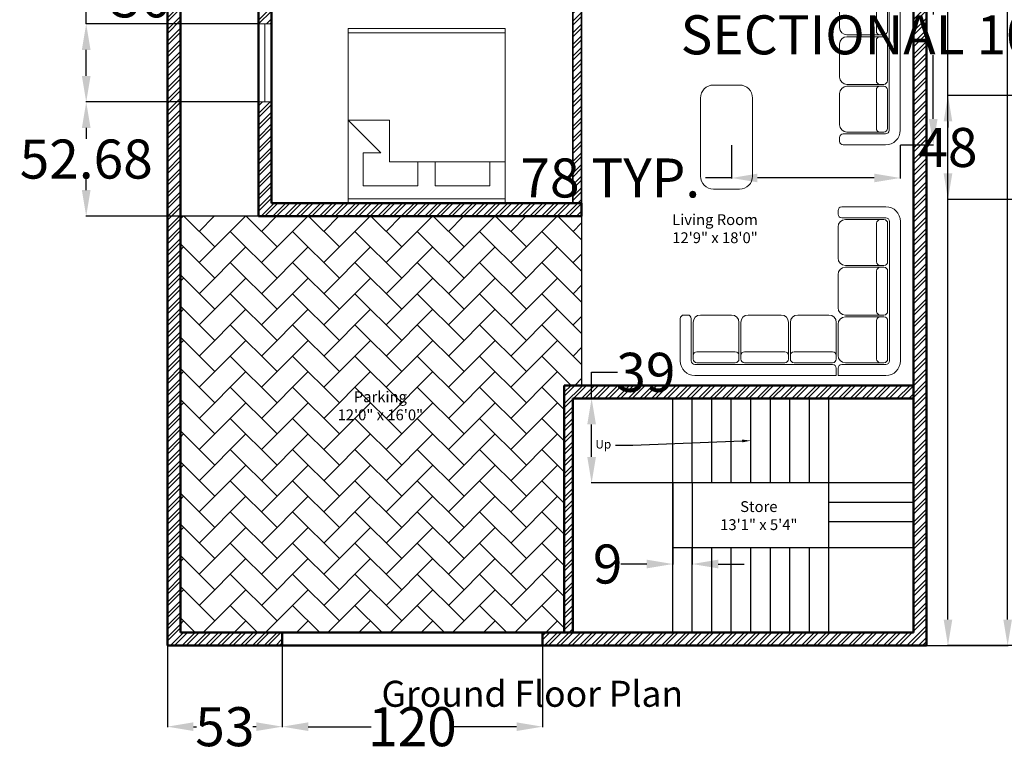
# Model space of a CAD drawing. Units: inches. Extents: x 73 to 1216, y -495 to 328.
# Tile 1 of 9: x 115 to 569, y -477 to -139. Entities that reach past the tile are written whole.
import ezdxf
from ezdxf import colors
from ezdxf.entities.mleader import LeaderData, LeaderLine
from ezdxf.math import Vec2, Vec3

# ---------------------------------------------------------------- set-up
doc = ezdxf.new("R2010")
doc.units = ezdxf.units.IN
for name, color, linetype, lineweight in [('A-ANNO-DIMS', 2, 'Continuous', 18), ('A-ANNO-TITL', 7, 'Continuous', 35), ('A-AREA-IDEN', 7, 'Continuous', 18), ('A-FLOR-EDGE', 7, 'Continuous', 25), ('A-FLOR-PATT', 9, 'Continuous', 13), ('A-GLAZ', 3, 'Continuous', 18), ('A-WALL-PATT', 8, 'Continuous', 13), ('Furniture', 2, 'Continuous', 18), ('Inner Walls', 5, 'Continuous', 35), ('Outer Walls', 1, 'Continuous', 50), ('Stairs', 8, 'Continuous', 25), ('Text-T18', 7, 'Continuous', 18)]:
    doc.layers.add(name, color=color, linetype=linetype, lineweight=lineweight)
doc.styles.get("Standard").update_dxf_attribs({"font": 'arial.ttf'})
doc.dimstyles.get("Standard").update_dxf_attribs({"dimtxt": 18, "dimasz": 12, "dimexe": 0.18, "dimexo": 0.0625, "dimgap": 0.09, "dimtad": 0, "dimtih": 1, "dimtoh": 1, "dimdec": 0, "dimzin": 0, "dimdsep": 46, "dimlunit": 3, "dimtxsty": 'Standard', "dimcen": 0.09, "dimadec": 0, "dimazin": 0, "dimtfac": 1, "dimtdec": 0, "dimtofl": 0, "dimtmove": 0, "dimatfit": 3, "dimfxl": 1, "dimtolj": 1, "dimtzin": 0, "dimarcsym": 0})
pattern_1 = [(45, (-434.707, -1257.0093), (-2.694077, 2.694077), []), (45, (-432.911, -1257.0093), (-2.694077, 2.694077), [])]

# ---------------------------------------------------------------- blocks, each defined once
blk = doc.blocks.new('KING-00')
for p, q in [((-0.897, -0.947), (-0.897, 0.882)), ((0.602, 0.882), (0.602, -0.464)), ((1.034, -0.947), (1.034, 0.882)), ((0.602, 0.704), (0.881, 0.704)), ((0.881, 0.069), (0.881, 0.704)), ((0.602, 0.069), (0.881, 0.069)), ((0.881, -0.134), (0.602, -0.134)), ((0.881, -0.769), (0.881, -0.134)), ((0.119, -0.464), (0.119, -0.947)), ((0.602, -0.464), (0.119, -0.464)), ((0.119, -0.947), (0.5, -0.566)), ((0.5, -0.769), (0.5, -0.566)), ((0.5, -0.769), (0.881, -0.769))]:
    blk.add_line(p, q)
blk.add_lwpolyline([(-0.948, -0.947), (-0.948, 0.882), (1.084, 0.882), (1.084, -0.947)], close=True)
blk = doc.blocks.new('A$C2AFA021D')
for p, q in [((0.8, 2.3), (0.2, 2.3)), ((0.2, 2.15), (0.8, 2.15)), ((0.85, 2.2), (0.85, 2.25)), ((0, 2.1), (0, 0.2)), ((0.15, 0.2), (0.15, 2.1)), ((0.175, 1.55), (0.175, 2.075)), ((0.225, 2.125), (0.275, 2.125)), ((0.75, 2.125), (0.275, 2.125)), ((0.325, 2.075), (0.325, 1.55)), ((0.85, 1.6), (0.85, 2.025)), ((0.275, 1.5), (0.225, 1.5)), ((0.275, 1.5), (0.75, 1.5)), ((0.175, 0.875), (0.175, 1.425)), ((0.225, 1.475), (0.275, 1.475)), ((0.75, 1.475), (0.275, 1.475)), ((0.325, 1.425), (0.325, 0.875)), ((0.85, 0.925), (0.85, 1.375)), ((0.275, 0.825), (0.225, 0.825)), ((0.275, 0.825), (0.75, 0.825)), ((0.975, 0.825), (1.4, 0.825)), ((1.625, 0.825), (2.075, 0.825)), ((2.3, 0.825), (2.725, 0.825)), ((2.9, 0.825), (2.95, 0.825)), ((0.175, 0.225), (0.175, 0.75)), ((0.225, 0.8), (0.275, 0.8)), ((0.75, 0.8), (0.275, 0.8)), ((0.325, 0.75), (0.325, 0.225)), ((0.85, 0.275), (0.85, 0.7)), ((0.875, 0.275), (0.875, 0.725)), ((1.5, 0.725), (1.5, 0.275)), ((1.525, 0.275), (1.525, 0.725)), ((2.175, 0.725), (2.175, 0.275)), ((2.2, 0.275), (2.2, 0.725)), ((2.825, 0.725), (2.825, 0.275)), ((2.85, 0.2), (2.85, 0.775)), ((3, 0.775), (3, 0.2)), ((0.875, 0.275), (0.875, 0.225)), ((1.45, 0.325), (0.925, 0.325)), ((1.5, 0.225), (1.5, 0.275)), ((1.525, 0.275), (1.525, 0.225)), ((2.125, 0.325), (1.575, 0.325)), ((2.175, 0.225), (2.175, 0.275)), ((2.2, 0.275), (2.2, 0.225)), ((2.775, 0.325), (2.25, 0.325)), ((2.825, 0.225), (2.825, 0.275)), ((0.8, 0.15), (0.2, 0.15)), ((0.275, 0.175), (0.225, 0.175)), ((0.275, 0.175), (0.75, 0.175)), ((0.925, 0.175), (1.45, 0.175)), ((0.925, 0.15), (2.8, 0.15)), ((1.575, 0.175), (2.125, 0.175)), ((2.25, 0.175), (2.775, 0.175)), ((0.85, 0), (0.85, 0.1)), ((0.875, 0.1), (0.875, 0)), ((0.2, 0), (0.85, 0)), ((2.8, 0), (0.875, 0))]:
    blk.add_line(p, q)
for centre, radius, start, end in [((0.2, 2.1), 0.2, 90, 180), ((0.8, 2.25), 0.05, 0, 90), ((0.2, 2.1), 0.05, 90, 180), ((0.8, 2.2), 0.05, 270, 0), ((0.225, 2.075), 0.05, 90, 180), ((0.275, 2.075), 0.05, 0, 90), ((0.75, 2.025), 0.1, 0, 90), ((0.225, 1.55), 0.05, 180, 270), ((0.275, 1.55), 0.05, 270, 0), ((0.75, 1.6), 0.1, 270, 0), ((0.225, 1.425), 0.05, 90, 180), ((0.275, 1.425), 0.05, 0, 90), ((0.75, 1.375), 0.1, 360, 90), ((0.225, 0.875), 0.05, 180, 270), ((0.275, 0.875), 0.05, 270, 0), ((0.75, 0.925), 0.1, 270, 0), ((0.975, 0.725), 0.1, 90, 180), ((1.4, 0.725), 0.1, 0, 90), ((1.625, 0.725), 0.1, 90, 180), ((2.075, 0.725), 0.1, 0, 90), ((2.3, 0.725), 0.1, 90, 180), ((2.725, 0.725), 0.1, 0, 90), ((2.9, 0.775), 0.05, 90, 180), ((2.95, 0.775), 0.05, 0, 90), ((0.225, 0.75), 0.05, 90, 180), ((0.275, 0.75), 0.05, 0, 90), ((0.75, 0.7), 0.1, 0, 90), ((0.75, 0.275), 0.1, 270, 0), ((0.925, 0.275), 0.05, 90, 180), ((1.45, 0.275), 0.05, 360, 90), ((1.575, 0.275), 0.05, 90, 180), ((2.125, 0.275), 0.05, 360, 90), ((2.25, 0.275), 0.05, 90, 180), ((2.775, 0.275), 0.05, 360, 90), ((0.2, 0.2), 0.2, 180, 270), ((0.2, 0.2), 0.05, 180, 270), ((0.225, 0.225), 0.05, 180, 270), ((0.275, 0.225), 0.05, 270, 0), ((0.8, 0.1), 0.05, 0, 90), ((0.925, 0.225), 0.05, 180, 270), ((0.925, 0.1), 0.05, 90, 180), ((1.45, 0.225), 0.05, 270, 0), ((1.575, 0.225), 0.05, 180, 270), ((2.125, 0.225), 0.05, 270, 0), ((2.25, 0.225), 0.05, 180, 270), ((2.775, 0.225), 0.05, 270, 0), ((2.8, 0.2), 0.2, 270, 0), ((2.8, 0.2), 0.05, 270, 0)]:
    blk.add_arc(centre, radius, start, end)
blk = doc.blocks.new('*U15')
for p, q in [((0, 6), (0, 0)), ((36, 6), (36, 0)), ((0, 3), (36, 3))]:
    blk.add_line(p, q)
blk = doc.blocks.new('STAIR-RETURN')
for p, q in [((0, 69), (0, 108)), ((9, 69), (9, 108)), ((18, 69), (18, 108)), ((27, 69), (27, 108)), ((36, 69), (36, 108)), ((45, 69), (45, 108)), ((54, 69), (54, 108)), ((63, 69), (63, 108)), ((72, 0), (72, 108)), ((111, 69), (0, 69)), ((0, 0), (0, 69)), ((111, 60), (72, 60)), ((111, 51), (72, 51)), ((111, 39), (0, 39)), ((9, 0), (9, 39)), ((18, 0), (18, 39)), ((27, 0), (27, 39)), ((36, 0), (36, 39)), ((45, 0), (45, 39)), ((54, 0), (54, 39)), ((63, 0), (63, 39))]:
    blk.add_line(p, q)
blk = doc.blocks.new('*D28')
at = {"layer": 'A-ANNO-DIMS', "color": 0, "lineweight": -2, "transparency": 16777216}
for p, q in [((520.8, -95.45), (536.15, -95.45)), ((535.97, -107.45), (535.97, -136.81)), ((535.97, -184.97), (535.97, -155.61)), ((520.8, -196.97), (536.15, -196.97))]:
    blk.add_line(p, q, dxfattribs=at)
at = {"layer": 'A-ANNO-DIMS', "color": 0, "transparency": 16777216}
for points in [[(533.97, -107.45), (537.97, -107.45), (535.97, -95.45)], [(533.97, -184.97), (537.97, -184.97), (535.97, -196.97)]]:
    blk.add_solid(points, dxfattribs=at)
at = {"layer": 'Defpoints', "color": 0, "transparency": 16777216}
for p in [(520.74, -95.45), (520.74, -196.97), (535.97, -196.97)]:
    blk.add_point(p, dxfattribs=at)
at = {"layer": 'A-ANNO-DIMS', "color": 0, "transparency": 16777216, "insert": (535.97, -146.21), "char_height": 18, "attachment_point": 5}
blk.add_mtext('\\A1;SECTIONAL 102 TYP.', dxfattribs=at)
blk = doc.blocks.new('*D29')
at = {"layer": 'A-ANNO-DIMS', "color": 0, "lineweight": -2, "transparency": 16777216}
for p, q in [((442.91, -197.03), (442.91, -212.38)), ((520.74, -197.03), (520.74, -212.38)), ((442.91, -212.2), (430.91, -212.2)), ((508.74, -212.2), (454.91, -212.2))]:
    blk.add_line(p, q, dxfattribs=at)
at = {"layer": 'A-ANNO-DIMS', "color": 0, "transparency": 16777216}
for points in [[(454.91, -210.2), (454.91, -214.2), (442.91, -212.2)], [(508.74, -210.2), (508.74, -214.2), (520.74, -212.2)]]:
    blk.add_solid(points, dxfattribs=at)
at = {"layer": 'Defpoints', "color": 0, "transparency": 16777216}
for p in [(442.91, -196.97), (520.74, -196.97), (442.91, -212.2)]:
    blk.add_point(p, dxfattribs=at)
at = {"layer": 'A-ANNO-DIMS', "color": 0, "transparency": 16777216, "insert": (387.08, -212.2), "char_height": 18, "attachment_point": 5}
blk.add_mtext('\\A1;78 TYP.', dxfattribs=at)
blk = doc.blocks.new('*D51')
at = {"layer": 'A-ANNO-DIMS', "color": 0, "lineweight": -2, "transparency": 16777216}
for p, q in [((532.94, 279.18), (570.45, 279.18)), ((570.27, 267.18), (570.27, -65.04)), ((570.27, -415.82), (570.27, -83.6)), ((532.94, -427.82), (570.45, -427.82))]:
    blk.add_line(p, q, dxfattribs=at)
at = {"layer": 'A-ANNO-DIMS', "color": 0, "transparency": 16777216}
for points in [[(568.27, 267.18), (572.27, 267.18), (570.27, 279.18)], [(568.27, -415.82), (572.27, -415.82), (570.27, -427.82)]]:
    blk.add_solid(points, dxfattribs=at)
at = {"layer": 'Defpoints', "color": 0, "transparency": 16777216}
for p in [(532.87, 279.18), (570.27, 279.18), (532.87, -427.82)]:
    blk.add_point(p, dxfattribs=at)
at = {"layer": 'A-ANNO-DIMS', "color": 0, "transparency": 16777216, "insert": (570.27, -74.32), "char_height": 18, "attachment_point": 5}
blk.add_mtext('\\A1;707', dxfattribs=at)
blk = doc.blocks.new('*D53')
at = {"layer": 'A-ANNO-DIMS', "color": 0, "lineweight": -2, "transparency": 16777216}
for p, q in [((580.1, 279.18), (542.58, 279.18)), ((542.76, 267.18), (542.76, -65.04)), ((542.76, -415.82), (542.76, -83.6)), ((580.1, -427.82), (542.58, -427.82))]:
    blk.add_line(p, q, dxfattribs=at)
at = {"layer": 'A-ANNO-DIMS', "color": 0, "transparency": 16777216}
for points in [[(540.76, 267.18), (544.76, 267.18), (542.76, 279.18)], [(540.76, -415.82), (544.76, -415.82), (542.76, -427.82)]]:
    blk.add_solid(points, dxfattribs=at)
at = {"layer": 'Defpoints', "color": 0, "transparency": 16777216}
for p in [(542.76, 279.18), (580.16, 279.18), (580.16, -427.82)]:
    blk.add_point(p, dxfattribs=at)
at = {"layer": 'A-ANNO-DIMS', "color": 0, "transparency": 16777216, "insert": (542.76, -74.32), "char_height": 18, "attachment_point": 5}
blk.add_mtext('\\A1;707', dxfattribs=at)
blk = doc.blocks.new('*D55')
at = {"layer": 'A-ANNO-DIMS', "color": 0, "lineweight": -2, "transparency": 16777216}
for p, q in [((235.87, -427.89), (235.87, -465.4)), ((355.87, -427.89), (355.87, -465.4)), ((247.87, -465.22), (276.78, -465.22)), ((343.87, -465.22), (314.97, -465.22))]:
    blk.add_line(p, q, dxfattribs=at)
at = {"layer": 'A-ANNO-DIMS', "color": 0, "transparency": 16777216}
for points in [[(247.87, -463.22), (247.87, -467.22), (235.87, -465.22)], [(343.87, -463.22), (343.87, -467.22), (355.87, -465.22)]]:
    blk.add_solid(points, dxfattribs=at)
at = {"layer": 'Defpoints', "color": 0, "transparency": 16777216}
for p in [(235.87, -427.82), (355.87, -427.82), (355.87, -465.22)]:
    blk.add_point(p, dxfattribs=at)
at = {"layer": 'A-ANNO-DIMS', "color": 0, "transparency": 16777216, "insert": (295.87, -465.22), "char_height": 18, "attachment_point": 5}
blk.add_mtext('\\A1;120', dxfattribs=at)
blk = doc.blocks.new('*D56')
at = {"layer": 'A-ANNO-DIMS', "color": 0, "lineweight": -2, "transparency": 16777216}
for p, q in [((182.87, -427.89), (182.87, -465.4)), ((235.87, -427.89), (235.87, -465.4)), ((194.87, -465.22), (196.39, -465.22)), ((223.87, -465.22), (222.36, -465.22))]:
    blk.add_line(p, q, dxfattribs=at)
at = {"layer": 'A-ANNO-DIMS', "color": 0, "transparency": 16777216}
for points in [[(194.87, -463.22), (194.87, -467.22), (182.87, -465.22)], [(223.87, -463.22), (223.87, -467.22), (235.87, -465.22)]]:
    blk.add_solid(points, dxfattribs=at)
at = {"layer": 'Defpoints', "color": 0, "transparency": 16777216}
for p in [(182.87, -427.82), (235.87, -427.82), (235.87, -465.22)]:
    blk.add_point(p, dxfattribs=at)
at = {"layer": 'A-ANNO-DIMS', "color": 0, "transparency": 16777216, "insert": (209.37, -465.22), "char_height": 18, "attachment_point": 5}
blk.add_mtext('\\A1;53', dxfattribs=at)
blk = doc.blocks.new('*D64')
at = {"layer": 'A-ANNO-DIMS', "color": 0, "lineweight": -2, "transparency": 16777216}
for p, q in [((145.47, -141.15), (145.47, -129.15)), ((145.47, -129.15), (157.47, -129.15)), ((224.81, -141.15), (145.29, -141.15)), ((145.47, -165.15), (145.47, -153.15)), ((224.81, -177.15), (145.29, -177.15))]:
    blk.add_line(p, q, dxfattribs=at)
at = {"layer": 'A-ANNO-DIMS', "color": 0, "transparency": 16777216}
for points in [[(143.47, -153.15), (147.47, -153.15), (145.47, -141.15)], [(143.47, -165.15), (147.47, -165.15), (145.47, -177.15)]]:
    blk.add_solid(points, dxfattribs=at)
at = {"layer": 'Defpoints', "color": 0, "transparency": 16777216}
for p in [(145.47, -141.15), (224.87, -141.15), (224.87, -177.15)]:
    blk.add_point(p, dxfattribs=at)
at = {"layer": 'A-ANNO-DIMS', "color": 0, "transparency": 16777216, "insert": (170.44, -129.15), "char_height": 18, "attachment_point": 5}
blk.add_mtext('\\A1;36', dxfattribs=at)
blk = doc.blocks.new('*D65')
at = {"layer": 'A-ANNO-DIMS', "color": 0, "lineweight": -2, "transparency": 16777216}
for p, q in [((224.81, -177.15), (145.29, -177.15)), ((145.47, -189.15), (145.47, -194.2)), ((145.47, -217.82), (145.47, -212.77)), ((224.81, -229.82), (145.29, -229.82))]:
    blk.add_line(p, q, dxfattribs=at)
at = {"layer": 'A-ANNO-DIMS', "color": 0, "transparency": 16777216}
for points in [[(143.47, -189.15), (147.47, -189.15), (145.47, -177.15)], [(143.47, -217.82), (147.47, -217.82), (145.47, -229.82)]]:
    blk.add_solid(points, dxfattribs=at)
at = {"layer": 'Defpoints', "color": 0, "transparency": 16777216}
for p in [(145.47, -177.15), (224.87, -177.15), (224.87, -229.82)]:
    blk.add_point(p, dxfattribs=at)
at = {"layer": 'A-ANNO-DIMS', "color": 0, "transparency": 16777216, "insert": (145.47, -203.49), "char_height": 18, "attachment_point": 5}
blk.add_mtext('\\A1;52.68', dxfattribs=at)
blk = doc.blocks.new('*D75')
at = {"layer": 'A-ANNO-DIMS', "color": 0, "lineweight": -2, "transparency": 16777216}
for p, q in [((378.47, -313.82), (378.47, -301.82)), ((378.47, -301.82), (390.47, -301.82)), ((415.81, -313.82), (378.29, -313.82)), ((378.47, -340.82), (378.47, -325.82)), ((415.81, -352.82), (378.29, -352.82))]:
    blk.add_line(p, q, dxfattribs=at)
at = {"layer": 'A-ANNO-DIMS', "color": 0, "transparency": 16777216}
for points in [[(376.47, -325.82), (380.47, -325.82), (378.47, -313.82)], [(376.47, -340.82), (380.47, -340.82), (378.47, -352.82)]]:
    blk.add_solid(points, dxfattribs=at)
at = {"layer": 'Defpoints', "color": 0, "transparency": 16777216}
for p in [(378.47, -313.82), (415.87, -313.82), (415.87, -352.82)]:
    blk.add_point(p, dxfattribs=at)
at = {"layer": 'A-ANNO-DIMS', "color": 0, "transparency": 16777216, "insert": (403.47, -301.82), "char_height": 18, "attachment_point": 5}
blk.add_mtext('\\A1;39', dxfattribs=at)
blk = doc.blocks.new('*D76')
at = {"layer": 'A-ANNO-DIMS', "color": 0, "lineweight": -2, "transparency": 16777216}
for p, q in [((415.87, -352.89), (415.87, -390.4)), ((424.87, -352.89), (424.87, -390.4)), ((403.87, -390.22), (391.87, -390.22)), ((436.87, -390.22), (448.87, -390.22))]:
    blk.add_line(p, q, dxfattribs=at)
at = {"layer": 'A-ANNO-DIMS', "color": 0, "transparency": 16777216}
for points in [[(403.87, -388.22), (403.87, -392.22), (415.87, -390.22)], [(436.87, -388.22), (436.87, -392.22), (424.87, -390.22)]]:
    blk.add_solid(points, dxfattribs=at)
at = {"layer": 'Defpoints', "color": 0, "transparency": 16777216}
for p in [(415.87, -352.82), (424.87, -352.82), (415.87, -390.22)]:
    blk.add_point(p, dxfattribs=at)
at = {"layer": 'A-ANNO-DIMS', "color": 0, "transparency": 16777216, "insert": (385.87, -390.22), "char_height": 18, "attachment_point": 5}
blk.add_mtext('\\A1;9', dxfattribs=at)
blk = doc.blocks.new('*D78')
at = {"layer": 'A-ANNO-DIMS', "color": 0, "lineweight": -2, "transparency": 16777216}
for p, q in [((831.3, -174.14), (542.58, -174.14)), ((542.76, -186.14), (542.76, -188.86)), ((542.76, -210.14), (542.76, -207.42)), ((831.3, -222.14), (542.58, -222.14))]:
    blk.add_line(p, q, dxfattribs=at)
at = {"layer": 'A-ANNO-DIMS', "color": 0, "transparency": 16777216}
for points in [[(540.76, -186.14), (544.76, -186.14), (542.76, -174.14)], [(540.76, -210.14), (544.76, -210.14), (542.76, -222.14)]]:
    blk.add_solid(points, dxfattribs=at)
at = {"layer": 'Defpoints', "color": 0, "transparency": 16777216}
for p in [(542.76, -174.14), (831.36, -174.14), (831.36, -222.14)]:
    blk.add_point(p, dxfattribs=at)
at = {"layer": 'A-ANNO-DIMS', "color": 0, "transparency": 16777216, "insert": (542.76, -198.14), "char_height": 18, "attachment_point": 5}
blk.add_mtext('\\A1;48', dxfattribs=at)

msp = doc.modelspace()

# ---------------------------------------------------------------- hatches: boundary and pattern name
at = {"layer": 'A-FLOR-PATT'}
h = msp.add_hatch(dxfattribs=at)
h.set_pattern_fill('AR-HBONE', color=256, scale=0.1)
h.set_pattern_definition([(45, (-434.707, -1257.009), (0, 14.36841), [30.48, -10.16]), (135, (-427.523, -1249.825), (1e-15, 14.36841), [30.48, -10.16])])
h.paths.add_polyline_path([(373.8746, -229.8237), (224.8746, -229.8237), (188.8746, -229.8237), (188.8746, -421.8237), (365.8746, -421.8237), (365.8746, -307.8237), (373.8746, -307.8237)])
h.paths.add_polyline_path([(260.5323, -326.9101), (301.2515, -326.9101), (301.2515, -307.9009), (260.5323, -307.9009)], flags=24)
at = {"layer": 'A-WALL-PATT'}
h = msp.add_hatch(dxfattribs=at)
h.set_pattern_fill('ANSI32', color=256, scale=0.4)
h.set_pattern_definition(pattern_1)
h.paths.add_polyline_path([(526.8746, -307.8237), (365.8746, -307.8237), (365.8746, -421.8237), (369.8746, -421.8237), (369.8746, -313.8237), (526.8746, -313.8237)], flags=17)
h.paths.add_polyline_path([(532.8746, 279.1763), (182.8746, 279.1763), (182.8746, -427.8237), (235.8746, -427.8237), (235.8746, -421.8237), (188.8746, -421.8237), (188.8746, 273.1763), (526.8746, 273.1763), (526.8746, -421.8237), (355.8746, -421.8237), (355.8746, -427.8237), (532.8746, -427.8237)])
h.paths.add_polyline_path([(230.8746, 197.1763), (224.8746, 197.1763), (224.8746, 83.4706), (230.8746, 83.4706)], flags=17)
h = msp.add_hatch(dxfattribs=at)
h.set_pattern_fill('ANSI32', color=256, scale=0.4)
h.set_pattern_definition(pattern_1)
h.paths.add_polyline_path([(287.8746, 201.1763), (281.8746, 201.1763), (281.8746, 206.1763), (277.8746, 206.1763), (277.8746, 201.1763), (218.9775, 201.1763), (218.9775, 197.1763), (287.8746, 197.1763)])
h.paths.add_polyline_path([(194.9775, 201.1763), (188.8746, 201.1763), (188.8746, 197.1763), (194.9775, 197.1763)])
h.paths.add_polyline_path([(281.8746, 273.1763), (277.8746, 273.1763), (277.8746, 236.1763), (281.8746, 236.1763)])
h.paths.add_polyline_path([(420.8746, 201.1763), (374.8746, 201.1763), (374.8746, 273.1763), (370.8746, 273.1763), (370.8746, 249.1763), (370.8746, 201.1763), (323.8746, 201.1763), (323.8746, 197.1763), (369.8746, 197.1763), (369.8746, 58.1763), (373.8746, 58.1763), (373.8746, 197.1763), (420.8746, 197.1763)])
h.paths.add_polyline_path([(472.8746, 201.1763), (466.8746, 201.1763), (466.8746, 273.1763), (462.8746, 273.1763), (462.8746, 201.1763), (456.8746, 201.1763), (456.8746, 197.1763), (472.8746, 197.1763)])
h.paths.add_polyline_path([(526.8746, 201.1763), (502.8746, 201.1763), (502.8746, 197.1763), (526.8746, 197.1763)])
h.paths.add_polyline_path([(373.8746, 22.1763), (369.8746, 22.1763), (369.8746, 16.1763), (230.8746, 16.1763), (230.8746, 12.1763), (373.8746, 12.1763)])
h.paths.add_polyline_path([(318.8746, -17.8237), (230.8746, -17.8237), (230.8746, -21.8237), (314.8746, -21.8237), (314.8746, -27.8237), (318.8746, -27.8237)])
h.paths.add_polyline_path([(327.8746, -87.8237), (318.8746, -87.8237), (318.8746, -57.8237), (314.8746, -57.8237), (314.8746, -87.8237), (230.8746, -87.8237), (230.8746, -91.8237), (327.8746, -91.8237)])
h.paths.add_polyline_path([(379.8746, -87.8237), (363.8746, -87.8237), (363.8746, -91.8237), (369.8746, -91.8237), (369.8746, -223.8237), (373.8746, -223.8237), (373.8746, -91.8237), (379.8746, -91.8237)])
h.paths.add_polyline_path([(448.8746, -87.8237), (430.8746, -87.8237), (430.8746, -33.8237), (436.8746, -33.8237), (436.8746, -29.8237), (426.8746, -29.8237), (426.8746, -87.8237), (419.8746, -87.8237), (419.8746, -91.8237), (448.8746, -91.8237)])
h.paths.add_polyline_path([(526.8746, -87.8237), (508.8746, -87.8237), (508.8746, -91.8237), (526.8746, -91.8237)])
h.paths.add_polyline_path([(526.8746, -29.8237), (514.8746, -29.8237), (514.8746, -33.8237), (526.8746, -33.8237)])
h.paths.add_polyline_path([(478.8746, -29.8237), (466.8746, -29.8237), (466.8746, -33.8237), (478.8746, -33.8237)])
h = msp.add_hatch(dxfattribs=at)
h.set_pattern_fill('ANSI32', color=256, scale=0.4)
h.set_pattern_definition(pattern_1)
h.paths.add_polyline_path([(230.8746, -71.6985), (224.8746, -71.6985), (224.8746, -141.1467), (230.8746, -141.1467)])
h.paths.add_polyline_path([(230.8746, 47.4706), (224.8746, 47.4706), (224.8746, -47.6985), (230.8746, -47.6985)])
h.paths.add_polyline_path([(230.8746, -177.1467), (224.8746, -177.1467), (224.8746, -229.8237), (373.8746, -229.8237), (373.8746, -223.8237), (230.8746, -223.8237)])

# ---------------------------------------------------------------- linework, layer by layer
at = {"layer": 'A-FLOR-EDGE'}
for p, q in [((224.8746, -229.8237), (188.8746, -229.8237)), ((373.8746, -229.8237), (373.8746, -307.8237))]:
    msp.add_line(p, q, dxfattribs=at)
at = {"layer": 'Furniture'}
msp.add_lwpolyline([(434.6734, -169.3446), (446.6734, -169.3446, -0.41421356), (452.6734, -175.3446), (452.6734, -211.3446, -0.41421356), (446.6734, -217.3446), (434.6734, -217.3446, -0.41421356), (428.6734, -211.3446), (428.6734, -175.3446, -0.41421356)], format="xyb", close=True, dxfattribs=at)
at = {"layer": 'Inner Walls'}
for p, q in [((369.8746, -223.8237), (369.8746, -91.8237)), ((373.8746, -223.8237), (373.8746, -91.8237))]:
    msp.add_line(p, q, dxfattribs=at)
at = {"layer": 'Outer Walls'}
for p, q in [((182.8746, -427.8237), (182.8746, 279.1763)), ((532.8746, -427.8237), (532.8746, 279.1763)), ((188.8746, -421.8237), (188.8746, 273.1763)), ((526.8746, -421.8237), (526.8746, 273.1763)), ((224.8746, -229.8237), (224.8746, 197.1763)), ((230.8746, -223.8237), (230.8746, 197.1763)), ((373.8746, -223.8237), (230.8746, -223.8237)), ((373.8746, -223.8237), (373.8746, -229.8237)), ((373.8746, -229.8237), (224.8746, -229.8237)), ((526.8746, -307.8237), (365.8746, -307.8237)), ((365.8746, -421.8237), (365.8746, -307.8237)), ((526.8746, -313.8237), (369.8746, -313.8237)), ((369.8746, -421.8237), (369.8746, -313.8237)), ((526.8746, -421.8237), (188.8746, -421.8237)), ((235.8746, -427.8237), (235.8746, -421.8237)), ((355.8746, -427.8237), (355.8746, -421.8237)), ((532.8746, -427.8237), (182.8746, -427.8237))]:
    msp.add_line(p, q, dxfattribs=at)

# ---------------------------------------------------------------- block references
at = {"layer": 'A-GLAZ', "rotation": 270}
msp.add_blockref('*U15', (224.8746, -141.1467), dxfattribs=at)
at = {"layer": 'Furniture'}
for name, p, xscale, yscale, zscale, rotation in [('A$C2AFA021D', (520.7411, -95.4493), -33.84012530478223, 33.84012530478223, 33.84012530478223, 90), ('KING-00', (303.6644, -180.8748), 39.60249106241186, 39.60249106241186, 39.60249106241186, 270)]:
    msp.add_blockref(name, p, dxfattribs=dict(at, xscale=xscale, yscale=yscale, zscale=zscale, rotation=rotation))
at = {"layer": 'Furniture', "xscale": -33.84012530478223, "yscale": 33.84012530478223, "zscale": 33.84012530478223}
msp.add_blockref('A$C2AFA021D', (520.8625, -303.3147), dxfattribs=at)
at = {"layer": 'Stairs'}
msp.add_blockref('STAIR-RETURN', (415.8746, -421.8237), dxfattribs=at)

# ---------------------------------------------------------------- texts
at = {"layer": 'A-ANNO-TITL', "insert": (426.4861, -444.0461), "char_height": 12, "attachment_point": 3}
msp.add_mtext_dynamic_manual_height_columns('\\pxqc;{\\fTimes New Roman|b0|i0|c0|p18;Ground Floor Plan}', width=150.706371, gutter_width=12.5, heights=[0], dxfattribs=at)
at = {"layer": 'A-AREA-IDEN', "char_height": 5, "attachment_point": 3}
for s, insert in [('\\pxqc;{\\fTimes New Roman|b0|i0|c0|p18;Living Room\\P12\'9" x 18\'0"}', (459.9033, -228.9181)), ('\\pxqc;{\\fTimes New Roman|b0|i0|c0|p18;Parking\\P12\'0" x 16\'0"}', (305.6303, -310.6036)), ('\\pxqc;{\\fTimes New Roman|b0|i0|c0|p18;Store\\P13\'1" x 5\'4"}', (480.1082, -361.2366))]:
    msp.add_mtext_dynamic_manual_height_columns(s, width=49.101878, gutter_width=12.5, heights=[0], dxfattribs=dict(at, insert=insert))

# ---------------------------------------------------------------- dimensions: what is measured, and where the dimension line sits
at = {"layer": 'A-ANNO-DIMS'}
for base, p1, p2, angle, override, picture, middle in [((542.7647, 279.1763), (580.1647, -427.8237), (580.1647, 279.1763), 90, {"dimdec": 0, "dimlfac": 1, "dimrnd": 0, "dimzin": 0, "dimdsep": 46, "dimlunit": 2}, '*D53', (542.7647, -74.3237)), ((570.2746, 279.1763), (532.8746, -427.8237), (532.8746, 279.1763), 90, {"dimdec": 0, "dimlfac": 1, "dimrnd": 0, "dimzin": 0, "dimdsep": 46, "dimlunit": 2}, '*D51', (570.2746, -74.3237)), ((145.4746, -141.1467), (224.8746, -177.1467), (224.8746, -141.1467), 90, {"dimdec": 0, "dimlfac": 1, "dimrnd": 0, "dimzin": 0, "dimdsep": 46, "dimlunit": 2}, '*D64', (170.4446, -129.1467)), ((542.7647, -174.1414), (831.3578, -222.1414), (831.3578, -174.1414), 90, {"dimdec": 0, "dimlfac": 1, "dimrnd": 0, "dimzin": 0, "dimdsep": 46, "dimlunit": 2}, '*D78', (542.7647, -198.1414)), ((145.4746, -177.1467), (224.8746, -229.8237), (224.8746, -177.1467), 90, {"dimdec": 2, "dimlfac": 1, "dimrnd": 0, "dimzin": 0, "dimdsep": 46, "dimlunit": 2}, '*D65', (145.4746, -203.4852)), ((378.4746, -313.8237), (415.8746, -352.8237), (415.8746, -313.8237), 90, {"dimdec": 0, "dimlfac": 1, "dimrnd": 0, "dimzin": 0, "dimdsep": 46, "dimlunit": 2}, '*D75', (403.4691, -301.8237)), ((415.8746, -390.2237), (424.8746, -352.8237), (415.8746, -352.8237), 180, {"dimdec": 0, "dimlfac": 1, "dimrnd": 0, "dimzin": 0, "dimdsep": 46, "dimlunit": 2}, '*D76', (385.8665, -390.2237))]:
    dim = msp.add_linear_dim(base=base, p1=p1, p2=p2, angle=angle, dimstyle='Standard', override=override, dxfattribs=at)
    dim.commit()
    dim.dimension.update_dxf_attribs({"geometry": picture, "text_midpoint": middle})
for base, p1, p2, angle, text, picture, middle in [((535.9692, -196.9696), (520.7411, -95.4493), (520.7411, -196.9696), 270, 'SECTIONAL <> TYP.', '*D28', (535.9692, -146.2095)), ((442.9088, -212.1977), (520.7411, -196.9696), (442.9088, -196.9696), 180, '<> TYP.', '*D29', (387.0835, -212.1977))]:
    dim = msp.add_linear_dim(base=base, p1=p1, p2=p2, angle=angle, text=text, dimstyle='Standard', override={"dimdec": 0, "dimlfac": 1, "dimrnd": 0, "dimzin": 0, "dimdsep": 46, "dimlunit": 2}, dxfattribs=at)
    dim.commit()
    dim.dimension.update_dxf_attribs({"geometry": picture, "text_midpoint": middle})
for base, p1, p2, picture, middle in [((235.8746, -465.2237), (182.8746, -427.8237), (235.8746, -427.8237), '*D56', (209.3746, -465.2237)), ((355.8746, -465.2237), (235.8746, -427.8237), (355.8746, -427.8237), '*D55', (295.8746, -465.2237))]:
    dim = msp.add_linear_dim(base=base, p1=p1, p2=p2, dimstyle='Standard', override={"dimdec": 0, "dimlfac": 1, "dimrnd": 0, "dimzin": 0, "dimdsep": 46, "dimlunit": 2}, dxfattribs=at)
    dim.commit()
    dim.dimension.update_dxf_attribs({"geometry": picture, "text_midpoint": middle})

# ---------------------------------------------------------------- leaders
at = {"layer": 'Text-T18'}
ml = msp.add_multileader_mtext('Standard', dxfattribs=at)
ml.set_content('{\\fTimes New Roman|b0|i0|c0|p18;Up}', color=256)
ml.set_leader_properties()
ml.build(insert=Vec2(0, 0))
ctx = ml.context
ctx.base_point, ctx.plane_origin = Vec3(378.5482, -335.5898), Vec3(451.8746, -333.3237)
ctx.text_align_type = 2
notes = []
notes.append((ctx, [(0, (1, 1, 0), (397.5331, -335.5898), (-1, 0), 8, [(0, [(451.8746, -333.3237)], 0, [])])]))
ctx.mtext.insert, ctx.mtext.alignment, ctx.mtext.flow_direction = Vec3(387.5331, -332.9582), 3, 5
for ctx, leaders in notes:
    for number, flags, end, landing, length, lines in leaders:
        leader = LeaderData()
        leader.index, (leader.has_last_leader_line, leader.has_dogleg_vector, leader.attachment_direction) = number, flags
        leader.last_leader_point, leader.dogleg_vector, leader.dogleg_length = Vec3(end), Vec3(landing), length
        for number, points, colour, breaks in lines:
            line = LeaderLine()
            line.index, line.vertices, line.color, line.breaks = number, Vec3.list(points), colors.encode_raw_color(colour), breaks
            leader.lines.append(line)
        ctx.leaders.append(leader)

doc.saveas('drawing.dxf')
